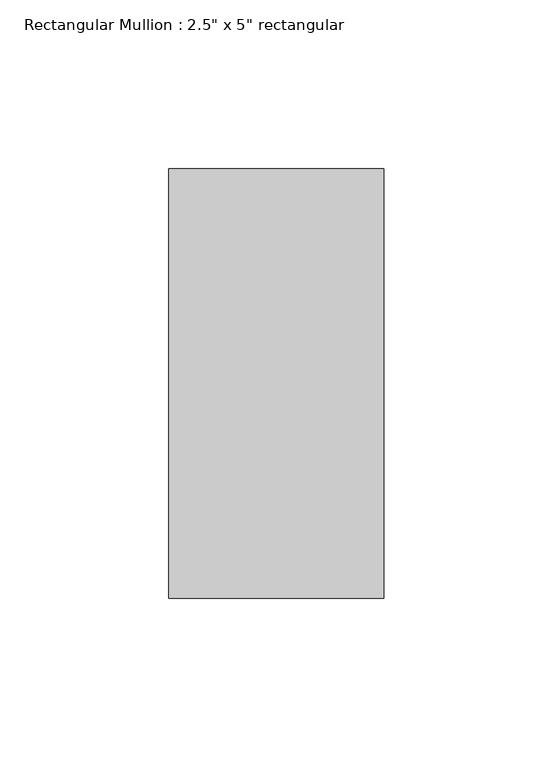
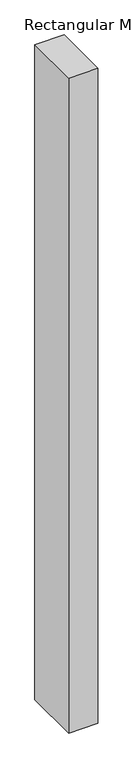
"""IFC4 building model written with IfcOpenShell, lengths in millimetres: member geometry."""

from ifc_helpers import new_model, si_unit, frame, origin, place, context, project, spatial, polyline, outline, extrude, source, transform, mapped, element, save


def member_9b0ed4fb(model_context):
    return source(origin(), model_context, "Body", "SweptSolid", [
        extrude(outline(polyline([(31.75, 63.5), (31.75, -63.5), (-31.75, -63.5), (-31.75, 63.5), (31.75, 63.5)])), frame((0.0, 0.0, -1503.5884629), z_axis=(0.0, 0.0, 1.0), x_axis=(1.0, 0.0, 0.0)), (0.0, 0.0, 1.0), 1503.5884629),
    ])


if __name__ == "__main__":
    model = new_model("IFC4")
    model_context = context("Model", 3, world=origin())
    ifc_project = project(units=[si_unit("LENGTHUNIT", "METRE", prefix="MILLI")], contexts=[model_context])
    site = spatial("IfcSite", under=ifc_project)
    building = spatial("IfcBuilding", under=site)
    placement = place(None, origin())
    member_shape = member_9b0ed4fb(model_context)
    element("IfcMember", 1, ObjectType="Rectangular Mullion : 2.5\" x 5\" rectangular", at=placement, inside=building, context=model_context, shape_type="MappedRepresentation", body=[
        mapped(member_shape, transform((0.0, 0.0, 0.0), x_axis=(1.0, 0.0, 0.0), y_axis=(0.0, 1.0, 0.0), z_axis=(0.0, 0.0, 1.0))),
    ])
    save(model, "model.ifc")

# Revit data of these elements
# Type "Rectangular Mullion : 2.5\" x 5\" rectangular"
#   built-in parameter 1007304 = 0.416667 (stored number, unit not read)
#   built-in parameter 1007301 = 0.104167 (stored number, unit not read)
#   built-in parameter 1007300 = 0.104167 (stored number, unit not read)
# Element 1 (IfcMember, "Rectangular Mullion : 2.5\" x 5\" rectangular")
#   Materials on its faces: "Aluminum"
# Materials
#   "Aluminum": class "Metal", colour RGB 247 247 247, transparency 0, Description = "Aluminum 6061", Cost = 0
